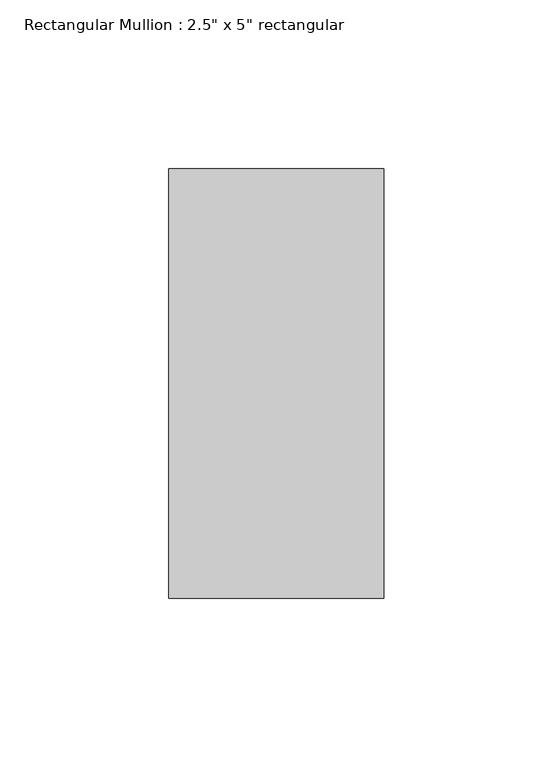
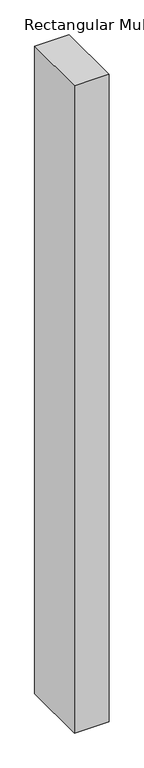
"""IFC4 building model written with IfcOpenShell, lengths in millimetres: member geometry."""

from ifc_helpers import new_model, si_unit, frame, origin, place, context, project, spatial, polyline, outline, extrude, source, transform, mapped, element, save


def member_8ea09a22(model_context):
    return source(origin(), model_context, "Body", "SweptSolid", [
        extrude(outline(polyline([(31.75, 63.5), (31.75, -63.5), (-31.75, -63.5), (-31.75, 63.5), (31.75, 63.5)])), frame((0.0, 0.0, -1260.0620128), z_axis=(0.0, 0.0, 1.0), x_axis=(1.0, 0.0, 0.0)), (0.0, 0.0, 1.0), 1260.0620128),
    ])


if __name__ == "__main__":
    model = new_model("IFC4")
    model_context = context("Model", 3, world=origin())
    ifc_project = project(units=[si_unit("LENGTHUNIT", "METRE", prefix="MILLI")], contexts=[model_context])
    site = spatial("IfcSite", under=ifc_project)
    building = spatial("IfcBuilding", under=site)
    placement = place(None, origin())
    member_shape = member_8ea09a22(model_context)
    element("IfcMember", 1, ObjectType="Rectangular Mullion : 2.5\" x 5\" rectangular", at=placement, inside=building, context=model_context, shape_type="MappedRepresentation", body=[
        mapped(member_shape, transform((0.0, 0.0, 0.0), x_axis=(1.0, 0.0, 0.0), y_axis=(0.0, 1.0, 0.0), z_axis=(0.0, 0.0, 1.0))),
    ])
    save(model, "model.ifc")

# Revit data of these elements
# Type "Rectangular Mullion : 2.5\" x 5\" rectangular"
#   built-in parameter 1007304 = 0.416667 (stored number, unit not read)
#   built-in parameter 1007301 = 0.104167 (stored number, unit not read)
#   built-in parameter 1007300 = 0.104167 (stored number, unit not read)
# Element 1 (IfcMember, "Rectangular Mullion : 2.5\" x 5\" rectangular")
#   Materials on its faces: "Aluminum"
# Materials
#   "Aluminum": class "Metal", colour RGB 247 247 247, transparency 0, Description = "Aluminum 6061", Cost = 0
